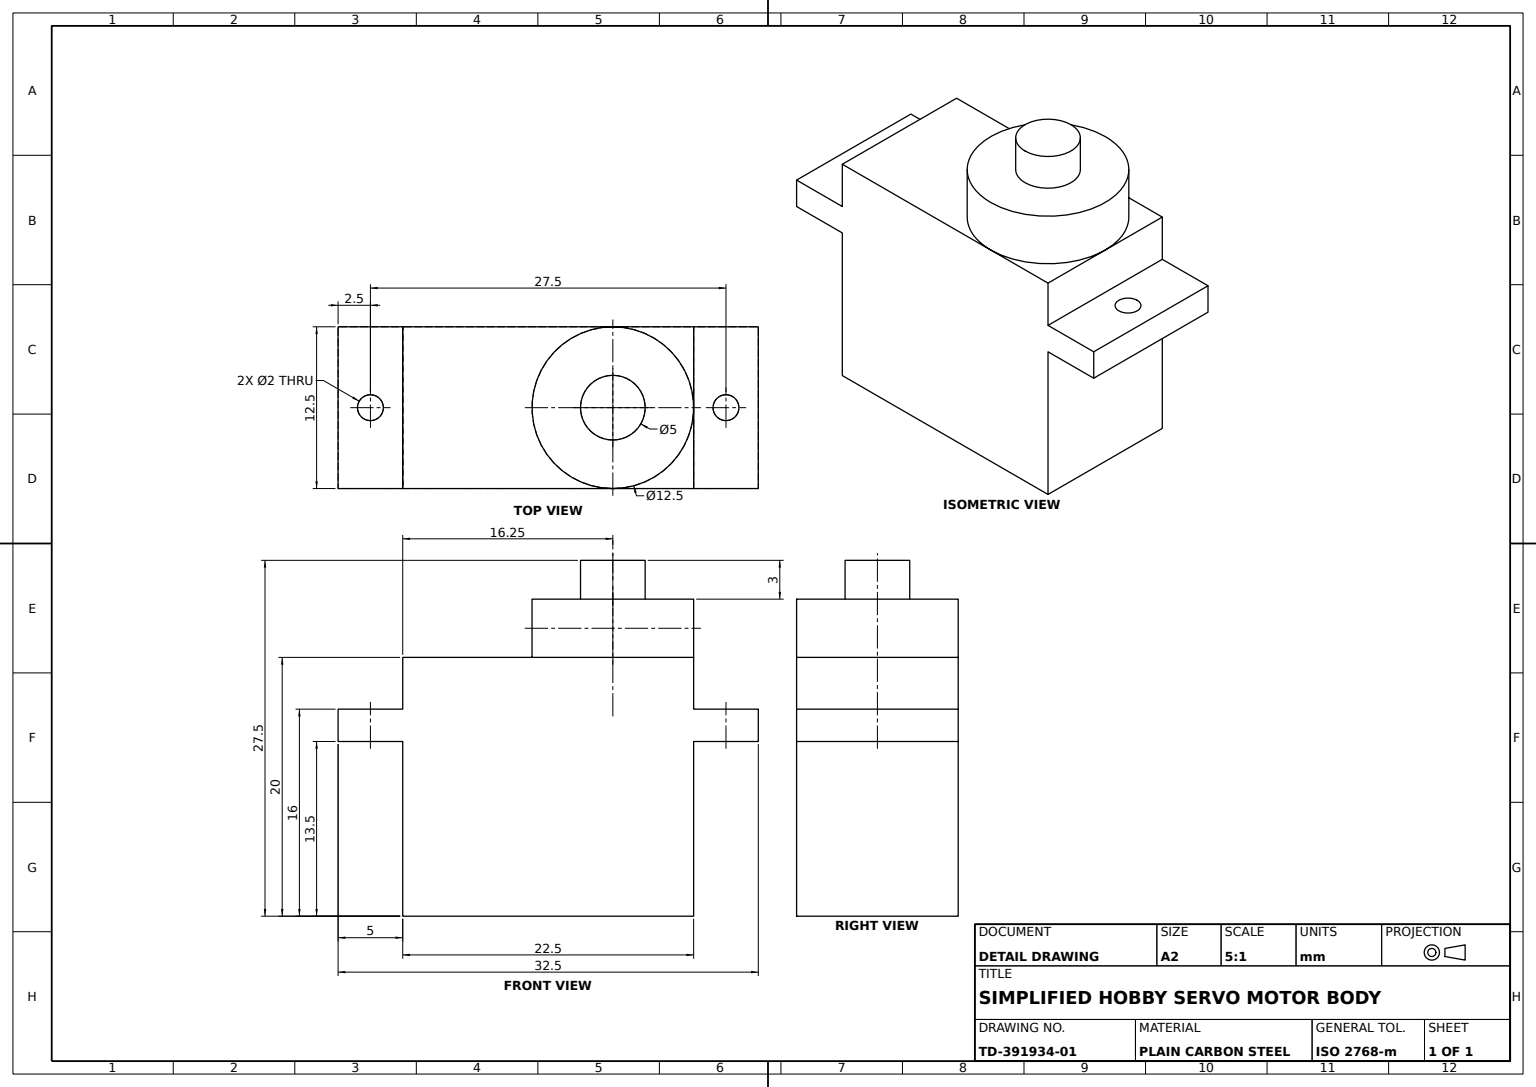
from build123d import *

# Parameters (mm, degrees)
SERVO_CASE_WITH_MOUNTING_TABS_DEPTH = 12.5
TAB_MOUNTING_HOLE_SKETCH_R          = 1
TAB_MOUNTING_HOLE_DEPTH             = 2.5
OUTPUT_GEAR_BOSS_SKETCH_12_5_R      = 6.25
OUTPUT_GEAR_BOSS_12_5_DEPTH         = 4.5
OUTPUT_SHAFT_SKETCH_5_R             = 2.5
OUTPUT_SHAFT_5_DEPTH                = 3


with BuildPart() as part:
    # Servo Case Profile Sketch → Servo Case with Mounting Tabs (new body)
    with BuildSketch(Plane.XY):
        Polygon((0, 0), (0, -4), (-5, -4), (-5, -6.5), (0, -6.5), (0, -20), (22.5, -20), (22.5, -6.5), (27.5, -6.5), (27.5, -4), (22.5, -4), (22.5, 0), align=None)
    extrude(amount=SERVO_CASE_WITH_MOUNTING_TABS_DEPTH)

    # Tab Mounting Hole Sketch → Tab Mounting Hole (cut)
    with BuildSketch(Plane(origin=(0, -4, 0), x_dir=(1, 0, 0), z_dir=(0, 1, 0))):
        with Locations(Location((25, -6.25, 0), (0, 0, 270))):
            Circle(TAB_MOUNTING_HOLE_SKETCH_R)
        with Locations(Location((-2.5, -6.25, 0), (0, 0, 270))):
            Circle(TAB_MOUNTING_HOLE_SKETCH_R)
    extrude(amount=-TAB_MOUNTING_HOLE_DEPTH, mode=Mode.SUBTRACT)

    # Output Gear Boss Sketch Ø12.5 → Output Gear Boss Ø12.5 (add)
    with BuildSketch(Plane(origin=(0, 0, 0), x_dir=(1, 0, 0), z_dir=(0, 1, 0))):
        with Locations(Location((16.25, -6.25, 0), (0, 0, 270))):
            Circle(OUTPUT_GEAR_BOSS_SKETCH_12_5_R)
    extrude(amount=OUTPUT_GEAR_BOSS_12_5_DEPTH)

    # Output Shaft Sketch Ø5 → Output Shaft Ø5 (add)
    with BuildSketch(Plane(origin=(0, 4.5, 0), x_dir=(1, 0, 0), z_dir=(0, 1, 0))):
        with Locations(Location((16.25, -6.25, 0), (0, 0, 270))):
            Circle(OUTPUT_SHAFT_SKETCH_5_R)
    extrude(amount=OUTPUT_SHAFT_5_DEPTH)


solid = part.part
